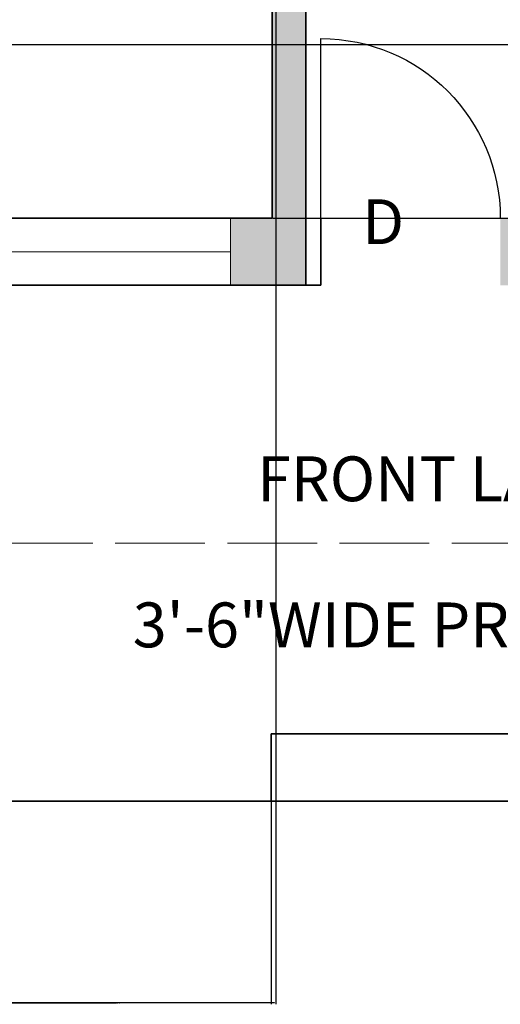
# Model space of a CAD drawing. Units: inches. Extents: x -5 to 330, y -522 to 40.
# Tile 7 of 23: x 95 to 159, y -522 to -391. Entities that reach past the tile are written whole.
import ezdxf

# ---------------------------------------------------------------- set-up
doc = ezdxf.new("R2010")
doc.units = ezdxf.units.IN
doc.header["$MEASUREMENT"] = 0
doc.linetypes.add('ACAD_ISO02W100', pattern=[15, 12, -3])
for name, color, linetype, lineweight in [('A-ANNO-DIMS', 2, 'Continuous', 18), ('A-ANNO-TEXT', 7, 'Continuous', 18), ('A-AREA-IDEN', 7, 'Continuous', 25), ('A-DOOR', 4, 'Continuous', 25), ('A-FLOR-CASE', 8, 'Continuous', 25), ('A-GLAZ', 4, 'Continuous', 18), ('A-ROOF-OVHD', 8, 'ACAD_ISO02W100', 18), ('A-SITE-WALL', 7, 'Continuous', 35), ('A-WALL', 7, 'Continuous', 35)]:
    doc.layers.add(name, color=color, linetype=linetype, lineweight=lineweight)
doc.layers.add('A-WALL-PATT', color=18, linetype='Continuous', lineweight=13, true_color=0x000000)
doc.styles.get("Standard").update_dxf_attribs({"font": 'arial.ttf'})
doc.dimstyles.get("Standard").update_dxf_attribs({"dimtxt": 0.18, "dimasz": 0.18, "dimexe": 0.18, "dimexo": 0.0625, "dimgap": 0.09, "dimtad": 0, "dimtih": 1, "dimtoh": 1, "dimdec": 0, "dimzin": 0, "dimdsep": 46, "dimlunit": 3, "dimtxsty": 'Standard', "dimcen": 0.09, "dimadec": 0, "dimazin": 0, "dimtfac": 1, "dimtdec": 0, "dimtofl": 0, "dimtmove": 0, "dimatfit": 3, "dimfxl": 1, "dimtolj": 1, "dimtzin": 0, "dimarcsym": 0})

# ---------------------------------------------------------------- blocks, each defined once
blk = doc.blocks.new('DOOR-24IN-SWING')
blk.add_line((24, 0), (24, 24))
blk.add_arc((24, 0), 24, 90, 180)
blk = doc.blocks.new('WIN-60IN-GLAZ')
for p, q in [((0, 9), (60, 9)), ((0, 4.5), (60, 4.5)), ((60, 0), (0, 0))]:
    blk.add_line(p, q)
blk = doc.blocks.new('*D39')
at = {"layer": 'A-ANNO-DIMS', "color": 0, "lineweight": -2, "transparency": 16777216}
for p, q in [((32.51, -495.21), (32.51, -522.31)), ((128.36, -495.21), (128.36, -522.31)), ((32.69, -522.13), (80.11, -522.13)), ((128.18, -522.13), (80.76, -522.13))]:
    blk.add_line(p, q, dxfattribs=at)
at = {"layer": 'A-ANNO-DIMS', "color": 0, "transparency": 16777216}
for points in [[(32.69, -522.1), (32.69, -522.16), (32.51, -522.13)], [(128.18, -522.1), (128.18, -522.16), (128.36, -522.13)]]:
    blk.add_solid(points, dxfattribs=at)
at = {"layer": 'Defpoints', "color": 0, "transparency": 16777216}
for p in [(32.51, -495.14), (128.36, -495.14), (128.36, -522.13)]:
    blk.add_point(p, dxfattribs=at)
at = {"layer": 'A-ANNO-DIMS', "color": 0, "transparency": 16777216, "insert": (80.44, -522.13), "char_height": 0.18, "attachment_point": 5}
blk.add_mtext('\\A1;8\'-0"', dxfattribs=at)
blk = doc.blocks.new('*D41')
at = {"layer": 'A-ANNO-DIMS', "color": 0, "lineweight": -2, "transparency": 16777216}
for p, q in [((87.01, -246.71), (87.01, -522.31)), ((129.01, -246.71), (129.01, -522.31)), ((87.19, -522.13), (107.68, -522.13)), ((128.83, -522.13), (108.34, -522.13))]:
    blk.add_line(p, q, dxfattribs=at)
at = {"layer": 'A-ANNO-DIMS', "color": 0, "transparency": 16777216}
for points in [[(87.19, -522.1), (87.19, -522.16), (87.01, -522.13)], [(128.83, -522.1), (128.83, -522.16), (129.01, -522.13)]]:
    blk.add_solid(points, dxfattribs=at)
at = {"layer": 'Defpoints', "color": 0, "transparency": 16777216}
for p in [(87.01, -246.64), (129.01, -246.64), (129.01, -522.13)]:
    blk.add_point(p, dxfattribs=at)
at = {"layer": 'A-ANNO-DIMS', "color": 0, "transparency": 16777216, "insert": (108.01, -522.13), "char_height": 0.18, "attachment_point": 5}
blk.add_mtext('\\A1;3\'-6"', dxfattribs=at)
blk = doc.blocks.new('*D44')
at = {"layer": 'A-ANNO-DIMS', "color": 0, "lineweight": -2, "transparency": 16777216}
for p, q in [((128.57, -393.93), (308.17, -393.93)), ((307.99, -394.11), (307.99, -405.36)), ((307.99, -416.96), (307.99, -405.72)), ((128.57, -417.14), (308.17, -417.14))]:
    blk.add_line(p, q, dxfattribs=at)
at = {"layer": 'A-ANNO-DIMS', "color": 0, "transparency": 16777216}
for points in [[(307.96, -394.11), (308.02, -394.11), (307.99, -393.93)], [(307.96, -416.96), (308.02, -416.96), (307.99, -417.14)]]:
    blk.add_solid(points, dxfattribs=at)
at = {"layer": 'Defpoints', "color": 0, "transparency": 16777216}
for p in [(128.51, -393.93), (307.99, -393.93), (128.51, -417.14)]:
    blk.add_point(p, dxfattribs=at)
at = {"layer": 'A-ANNO-DIMS', "color": 0, "transparency": 16777216, "insert": (307.99, -405.54), "char_height": 0.18, "attachment_point": 5}
blk.add_mtext('\\A1;1\'-11"', dxfattribs=at)

msp = doc.modelspace()

# ---------------------------------------------------------------- hatches: boundary and pattern name
at = {"layer": 'A-WALL-PATT'}
h = msp.add_hatch(color=256, dxfattribs=at)
h.dxf.hatch_style = 1
h.paths.add_polyline_path([(164.01, -44.15), (159.51, -44.15), (159.51, -153.14), (164.01, -153.14)], flags=17)
h.paths.add_polyline_path([(224.01, -188.14), (272.01, -188.14), (272.01, -218.14), (260.01, -218.14), (260.01, -222.64), (272.01, -222.64), (272.01, -292.64), (159.01, -292.64), (159.01, -297.14), (272.01, -297.14), (272.01, -417.14), (245.51, -417.14), (245.51, -426.14), (272.01, -426.14), (272.01, -495.14), (281.01, -495.14), (281.01, 12.36), (23.51, 12.36), (23.51, -426.14), (62.92, -426.14), (62.92, -417.14), (32.51, -417.14), (32.51, -297.14), (48.13, -297.14), (48.13, -292.64), (32.51, -292.64), (32.51, -140.64), (133.51, -140.64), (133.51, -131.64), (32.51, -131.64), (32.51, 3.36), (159.51, 3.36), (164.01, 3.36), (220.01, 3.36), (224.51, 3.36), (272.01, 3.36), (272.01, -179.14), (159.51, -179.14), (159.51, -188.14), (219.51, -188.14), (219.51, -266.64), (224.01, -266.64), (224.01, -222.64), (236.01, -222.64), (236.01, -218.14), (224.01, -218.14)])
h.paths.add_polyline_path([(133.01, -292.64), (128.51, -292.64), (128.51, -297.14), (128.51, -417.14), (122.92, -417.14), (122.92, -426.14), (133.01, -426.14)], flags=17)
h.paths.add_polyline_path([(185.51, -417.14), (159.01, -417.14), (159.01, -426.14), (185.51, -426.14)], flags=17)
h.paths.add_polyline_path([(133.51, -140.64), (129.01, -140.64), (129.01, -246.64), (133.51, -246.64)], flags=17)
h.paths.add_polyline_path([(246.01, -48.64), (224.51, -48.64), (224.51, -27.63), (220.01, -27.63), (220.01, -48.64), (198.6, -48.64), (198.6, -53.14), (246.01, -53.14)], flags=17)

# ---------------------------------------------------------------- linework, layer by layer
at = {"layer": 'A-FLOR-CASE'}
msp.add_line((48.13, -393.93), (128.51, -393.93), dxfattribs=at)
at = {"layer": 'A-GLAZ'}
msp.add_line((122.92, -417.14), (122.92, -426.14), dxfattribs=at)
at = {"layer": 'A-ROOF-OVHD'}
msp.add_line((32.51, -460.64), (272.01, -460.64), dxfattribs=at)
at = {"layer": 'A-SITE-WALL'}
for p, q in [((128.36, -486.14), (272.01, -486.14)), ((128.36, -486.14), (128.36, -495.14)), ((23.51, -495.14), (281.01, -495.14))]:
    msp.add_line(p, q, dxfattribs=at)
at = {"layer": 'A-WALL'}
for p, q in [((133.01, -292.64), (133.01, -426.14)), ((128.51, -297.14), (128.51, -417.14)), ((32.51, -417.14), (128.51, -417.14)), ((135.01, -426.14), (135.01, -417.14)), ((23.51, -426.14), (135.01, -426.14))]:
    msp.add_line(p, q, dxfattribs=at)

# ---------------------------------------------------------------- block references
at = {"layer": 'A-DOOR', "extrusion": (0, 0, -1), "zscale": -1}
msp.add_blockref('DOOR-24IN-SWING', (-159.01, -417.14), dxfattribs=at)
at = {"layer": 'A-GLAZ'}
msp.add_blockref('WIN-60IN-GLAZ', (62.92, -426.14), dxfattribs=at)

# ---------------------------------------------------------------- texts
at = {"layer": 'A-ANNO-TEXT', "char_height": 6, "attachment_point": 1}
for s, insert in [('D', (140.52, -414.63)), ('3\'-6"WIDE PROJECTION', (109.86, -468.56))]:
    msp.add_mtext(s, dxfattribs=dict(at, insert=insert))
at = {"layer": 'A-AREA-IDEN', "insert": (126.49, -449.02), "char_height": 6, "attachment_point": 1}
msp.add_mtext('FRONT LAWN', dxfattribs=at)

# ---------------------------------------------------------------- dimensions: what is measured, and where the dimension line sits
at = {"layer": 'A-ANNO-DIMS'}
for base, p1, p2, picture, middle in [((129.01, -522.13), (87.01, -246.64), (129.01, -246.64), '*D41', (108.01, -522.13)), ((128.3612, -522.1286), (32.5099, -495.1436), (128.3612, -495.1436), '*D39', (80.4356, -522.1286))]:
    dim = msp.add_linear_dim(base=base, p1=p1, p2=p2, dimstyle='Standard', override={"dimdec": 1, "dimlfac": 1, "dimrnd": 0, "dimzin": 1, "dimdsep": 46, "dimlunit": 4, "dimfrac": 2}, dxfattribs=at)
    dim.commit()
    dim.dimension.update_dxf_attribs({"geometry": picture, "text_midpoint": middle})
dim = msp.add_linear_dim(base=(307.99, -393.93), p1=(128.51, -417.14), p2=(128.51, -393.93), angle=90, dimstyle='Standard', override={"dimdec": 1, "dimlfac": 1, "dimrnd": 0, "dimzin": 1, "dimdsep": 46, "dimlunit": 4, "dimfrac": 2}, dxfattribs=at)
dim.commit()
dim.dimension.update_dxf_attribs({"geometry": '*D44', "text_midpoint": (307.99, -405.54)})

doc.saveas('drawing.dxf')
